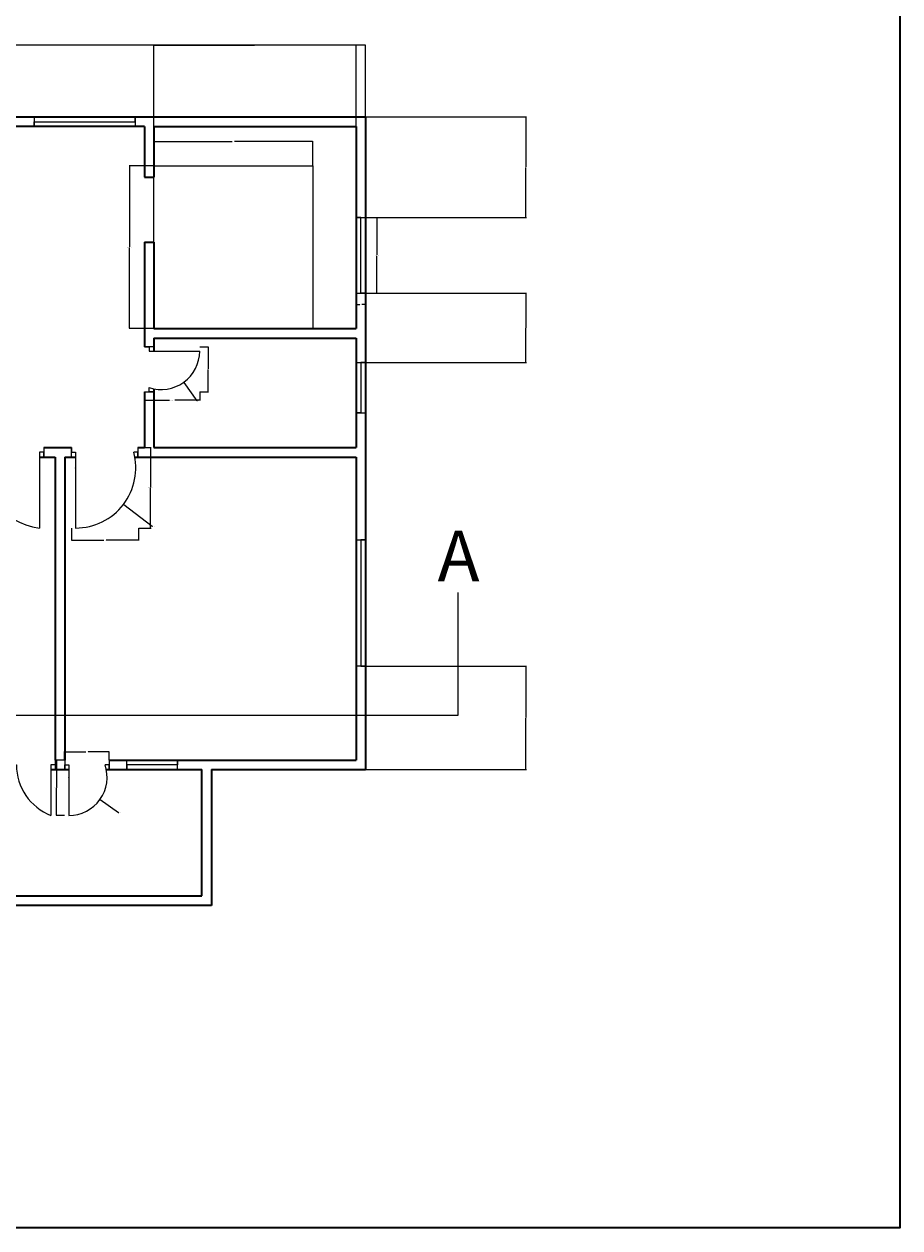
# Model space of a CAD drawing. Units: inches. Extents: x 2055 to 3558, y 1520 to 2888.
# Tile 6 of 8: x 3142 to 3558, y 1520 to 2092. Entities that reach past the tile are written whole.
import ezdxf

# ---------------------------------------------------------------- set-up
doc = ezdxf.new("R2010")
doc.units = ezdxf.units.IN
for name, color, linetype, lineweight in [('A-ANNO-DIMS', 2, 'Continuous', 18), ('A-ANNO-SYMB', 7, 'Continuous', 25), ('A-ANNO-TTLB', 7, 'Continuous', 35), ('A-DOOR', 3, 'Continuous', 18), ('A-FLOR-FIXT', 8, 'Continuous', 18), ('A-GLAZ', 4, 'Continuous', 18), ('A-WALL', 7, 'Continuous', 35)]:
    doc.layers.add(name, color=color, linetype=linetype, lineweight=lineweight)
doc.styles.get("Standard").update_dxf_attribs({"font": 'arial.ttf'})
doc.dimstyles.get("Standard").update_dxf_attribs({"dimtxt": 0.18, "dimasz": 0.18, "dimexe": 0.18, "dimexo": 0.0625, "dimgap": 0.09, "dimtad": 0, "dimtih": 1, "dimtoh": 1, "dimdec": 4, "dimzin": 0, "dimdsep": 46, "dimtxsty": 'Standard', "dimcen": 0.09, "dimadec": 0, "dimazin": 0, "dimtfac": 1, "dimtdec": 4, "dimtofl": 0, "dimtmove": 0, "dimatfit": 3, "dimfxl": 1, "dimtolj": 1, "dimtzin": 0, "dimarcsym": 0})

# ---------------------------------------------------------------- blocks, each defined once
blk = doc.blocks.new('DOOR-BATH-24-B')
for p, q in [((4.5, 21.32), (0, 21.32)), ((0, 21.32), (2.25, 21.32)), ((2.25, 21.32), (2.25, 19.32)), ((2.25, 19.32), (26.25, 19.32)), ((0, 0), (4.5, 0)), ((2.25, 0), (2.25, 2)), ((4.5, 0), (2.25, 0))]:
    blk.add_line(p, q)
blk.add_arc((8, 19.32), 18.25, 251.6403, 0)
blk = doc.blocks.new('DOOR-BED-36-F')
for p, q in [((0, 33.75), (0, 38.25)), ((0, 38.25), (0, 36)), ((0, 36), (2, 36)), ((2, 36), (2, 0)), ((31.57, 36), (29.57, 36)), ((31.57, 38.25), (31.57, 33.75)), ((31.57, 33.75), (31.57, 36))]:
    blk.add_line(p, q)
blk.add_arc((2, 28.56), 28.56, 270, 15.1117)
blk = doc.blocks.new('DOOR-BED-36-G')
for p, q in [((0, 38.25), (0, 33.75)), ((0, 33.75), (0, 36)), ((0, 36), (2, 36)), ((34.89, 36), (32.89, 36)), ((32.89, 36), (32.89, 0)), ((34.89, 38.25), (34.89, 33.75)), ((34.89, 33.75), (34.89, 36))]:
    blk.add_line(p, q)
blk.add_arc((38.42, 36), 36.42, 180, 261.253)
blk = doc.blocks.new('DOOR-VERANDA-24-A')
for p, q in [((0, 26.25), (0, 21.75)), ((0, 21.75), (0, 24)), ((0, 24), (2, 24)), ((2, 24), (2, 0)), ((21.18, 24), (19.18, 24)), ((21.18, 26.25), (21.18, 21.75)), ((21.18, 21.75), (21.18, 24))]:
    blk.add_line(p, q)
blk.add_arc((2, 18.15), 18.15, 270, 18.8194)
blk = doc.blocks.new('DOOR-VERANDA-24-B')
for p, q in [((0, 26.25), (0, 21.75)), ((0, 21.75), (0, 24)), ((0, 24), (2, 24)), ((20.42, 24), (18.42, 24)), ((18.42, 24), (18.42, 0)), ((20.42, 26.25), (20.42, 21.75))]:
    blk.add_line(p, q)
blk.add_arc((27.75, 24), 25.75, 180, 248.7547)
blk = doc.blocks.new('WIN-36')
for p, q in [((2.25, 36), (0, 36)), ((0, 36), (4.5, 36)), ((2.25, 0), (2.25, 36)), ((0, 0), (4.5, 0)), ((4.5, 0), (2.25, 0))]:
    blk.add_line(p, q)
blk = doc.blocks.new('WIN-24')
for p, q in [((0, 24), (4.5, 24)), ((4.5, 24), (2.25, 24)), ((2.25, 24), (2.25, 0)), ((2.25, 0), (0, 0)), ((0, 0), (4.5, 0))]:
    blk.add_line(p, q)
blk = doc.blocks.new('WIN-60-2')
for p, q in [((4.5, 60), (0, 60)), ((0, 60), (2.25, 60)), ((2.25, 60), (2.25, 0)), ((2.25, 0), (0, 0)), ((0, 0), (4.5, 0))]:
    blk.add_line(p, q)
blk = doc.blocks.new('WIN-48')
for p, q in [((0, 4.5), (0, 0)), ((0, 0), (0, 2.25)), ((0, 2.25), (48, 2.25)), ((48, 2.25), (48, 4.5)), ((48, 4.5), (48, 0))]:
    blk.add_line(p, q)
blk = doc.blocks.new('COUNTER-4')
for p, q in [((0, 77.26), (75.5, 77.26)), ((75.5, 77.26), (75.5, 0))]:
    blk.add_line(p, q)
blk = doc.blocks.new('VERANDA-PERIMETER')
for p, q in [((0, 0), (0, 64.5)), ((4.5, 64.5), (4.5, 4.5)), ((124.15, 4.5), (124.15, 64.5)), ((128.65, 64.5), (128.65, 4.5)), ((4.5, 0), (0, 0)), ((4.5, 4.5), (124.15, 4.5)), ((128.65, 0), (4.5, 0)), ((128.65, 4.5), (128.65, 0))]:
    blk.add_line(p, q)
blk = doc.blocks.new('*D42')
at = {"layer": 'A-ANNO-DIMS', "color": 0, "lineweight": -2, "transparency": 16777216}
for p, q in [((3304.06, 2000.28), (3309.58, 2000.28)), ((3309.4, 2000.1), (3309.4, 1982.46)), ((3309.4, 1964.46), (3309.4, 1982.1)), ((3304.06, 1964.28), (3309.58, 1964.28))]:
    blk.add_line(p, q, dxfattribs=at)
at = {"layer": 'A-ANNO-DIMS', "color": 0, "transparency": 16777216}
for points in [[(3309.37, 2000.1), (3309.43, 2000.1), (3309.4, 2000.28)], [(3309.37, 1964.46), (3309.43, 1964.46), (3309.4, 1964.28)]]:
    blk.add_solid(points, dxfattribs=at)
at = {"layer": 'Defpoints', "color": 0, "transparency": 16777216}
for p in [(3304, 2000.28), (3309.4, 2000.28), (3304, 1964.28)]:
    blk.add_point(p, dxfattribs=at)
at = {"layer": 'A-ANNO-DIMS', "color": 0, "transparency": 16777216, "insert": (3309.4, 1982.28), "char_height": 0.18, "attachment_point": 5}
blk.add_mtext('\\A1;WINDOW 36 TYP.', dxfattribs=at)
blk = doc.blocks.new('*D43')
at = {"layer": 'A-ANNO-DIMS', "color": 0, "lineweight": -2, "transparency": 16777216}
for p, q in [((3299.5, 1964.22), (3299.5, 1958.7)), ((3304, 1964.22), (3304, 1958.7)), ((3299.68, 1958.88), (3301.29, 1958.88)), ((3303.82, 1958.88), (3302.2, 1958.88))]:
    blk.add_line(p, q, dxfattribs=at)
at = {"layer": 'A-ANNO-DIMS', "color": 0, "transparency": 16777216}
for points in [[(3299.68, 1958.91), (3299.68, 1958.85), (3299.5, 1958.88)], [(3303.82, 1958.91), (3303.82, 1958.85), (3304, 1958.88)]]:
    blk.add_solid(points, dxfattribs=at)
at = {"layer": 'Defpoints', "color": 0, "transparency": 16777216}
for p in [(3299.5, 1964.28), (3304, 1964.28), (3304, 1958.88)]:
    blk.add_point(p, dxfattribs=at)
at = {"layer": 'A-ANNO-DIMS', "color": 0, "transparency": 16777216, "insert": (3301.75, 1958.88), "char_height": 0.18, "attachment_point": 5}
blk.add_mtext('\\A1;5 TYP.', dxfattribs=at)
blk = doc.blocks.new('*D68')
at = {"layer": 'A-ANNO-DIMS', "color": 0, "lineweight": -2, "transparency": 16777216}
for p, q in [((3199, 1917.43), (3199, 1913.38)), ((3225.25, 1917.43), (3225.25, 1913.38)), ((3199.18, 1913.56), (3210.81, 1913.56)), ((3225.07, 1913.56), (3213.43, 1913.56))]:
    blk.add_line(p, q, dxfattribs=at)
at = {"layer": 'A-ANNO-DIMS', "color": 0, "transparency": 16777216}
for points in [[(3199.18, 1913.59), (3199.18, 1913.53), (3199, 1913.56)], [(3225.07, 1913.59), (3225.07, 1913.53), (3225.25, 1913.56)]]:
    blk.add_solid(points, dxfattribs=at)
at = {"layer": 'Defpoints', "color": 0, "transparency": 16777216}
for p in [(3199, 1917.49), (3225.25, 1917.49), (3225.25, 1913.56)]:
    blk.add_point(p, dxfattribs=at)
at = {"layer": 'A-ANNO-DIMS', "color": 0, "transparency": 16777216, "insert": (3212.12, 1913.56), "char_height": 0.18, "attachment_point": 5}
blk.add_mtext('\\A1;BATH DOOR 26 TYP.', dxfattribs=at)
blk = doc.blocks.new('*D69')
at = {"layer": 'A-ANNO-DIMS', "color": 0, "lineweight": -2, "transparency": 16777216}
for p, q in [((3225.31, 1938.82), (3229.36, 1938.82)), ((3229.18, 1938.64), (3229.18, 1928.34)), ((3229.18, 1917.67), (3229.18, 1927.98)), ((3225.31, 1917.49), (3229.36, 1917.49))]:
    blk.add_line(p, q, dxfattribs=at)
at = {"layer": 'A-ANNO-DIMS', "color": 0, "transparency": 16777216}
for points in [[(3229.15, 1938.64), (3229.21, 1938.64), (3229.18, 1938.82)], [(3229.15, 1917.67), (3229.21, 1917.67), (3229.18, 1917.49)]]:
    blk.add_solid(points, dxfattribs=at)
at = {"layer": 'Defpoints', "color": 0, "transparency": 16777216}
for p in [(3225.25, 1938.82), (3229.18, 1938.82), (3225.25, 1917.49)]:
    blk.add_point(p, dxfattribs=at)
at = {"layer": 'A-ANNO-DIMS', "color": 0, "transparency": 16777216, "insert": (3229.18, 1928.16), "char_height": 0.18, "attachment_point": 5}
blk.add_mtext('\\A1;21 TYP.', dxfattribs=at)
blk = doc.blocks.new('*D78')
at = {"layer": 'A-ANNO-DIMS', "color": 0, "lineweight": -2, "transparency": 16777216}
for p, q in [((3196.25, 1891), (3202.11, 1891)), ((3201.93, 1890.82), (3201.93, 1872.06)), ((3201.93, 1852.93), (3201.93, 1871.69)), ((3196.25, 1852.75), (3202.11, 1852.75))]:
    blk.add_line(p, q, dxfattribs=at)
at = {"layer": 'A-ANNO-DIMS', "color": 0, "transparency": 16777216}
for points in [[(3201.9, 1890.82), (3201.96, 1890.82), (3201.93, 1891)], [(3201.9, 1852.93), (3201.96, 1852.93), (3201.93, 1852.75)]]:
    blk.add_solid(points, dxfattribs=at)
at = {"layer": 'Defpoints', "color": 0, "transparency": 16777216}
for p in [(3196.19, 1891), (3201.93, 1891), (3196.19, 1852.75)]:
    blk.add_point(p, dxfattribs=at)
at = {"layer": 'A-ANNO-DIMS', "color": 0, "transparency": 16777216, "insert": (3201.93, 1871.87), "char_height": 0.18, "attachment_point": 5}
blk.add_mtext('\\A1;BED DOOR 38 TYP.', dxfattribs=at)
blk = doc.blocks.new('*D79')
at = {"layer": 'A-ANNO-DIMS', "color": 0, "lineweight": -2, "transparency": 16777216}
for p, q in [((3164.3, 1852.69), (3164.3, 1846.83)), ((3196.19, 1852.69), (3196.19, 1846.83)), ((3164.48, 1847.01), (3179.72, 1847.01)), ((3196.01, 1847.01), (3180.77, 1847.01))]:
    blk.add_line(p, q, dxfattribs=at)
at = {"layer": 'A-ANNO-DIMS', "color": 0, "transparency": 16777216}
for points in [[(3164.48, 1847.04), (3164.48, 1846.98), (3164.3, 1847.01)], [(3196.01, 1847.04), (3196.01, 1846.98), (3196.19, 1847.01)]]:
    blk.add_solid(points, dxfattribs=at)
at = {"layer": 'Defpoints', "color": 0, "transparency": 16777216}
for p in [(3164.3, 1852.75), (3196.19, 1852.75), (3196.19, 1847.01)]:
    blk.add_point(p, dxfattribs=at)
at = {"layer": 'A-ANNO-DIMS', "color": 0, "transparency": 16777216, "insert": (3180.25, 1847.01), "char_height": 0.18, "attachment_point": 5}
blk.add_mtext('\\A1;32 TYP.', dxfattribs=at)
blk = doc.blocks.new('*D82')
at = {"layer": 'A-ANNO-DIMS', "color": 0, "lineweight": -2, "transparency": 16777216}
for p, q in [((3161.03, 1742.5), (3156.98, 1742.5)), ((3157.16, 1742.32), (3157.16, 1729.56)), ((3157.16, 1716.43), (3157.16, 1729.19)), ((3161.03, 1716.25), (3156.98, 1716.25))]:
    blk.add_line(p, q, dxfattribs=at)
at = {"layer": 'A-ANNO-DIMS', "color": 0, "transparency": 16777216}
for points in [[(3157.13, 1742.32), (3157.19, 1742.32), (3157.16, 1742.5)], [(3157.13, 1716.43), (3157.19, 1716.43), (3157.16, 1716.25)]]:
    blk.add_solid(points, dxfattribs=at)
at = {"layer": 'Defpoints', "color": 0, "transparency": 16777216}
for p in [(3157.16, 1742.5), (3161.09, 1742.5), (3161.09, 1716.25)]:
    blk.add_point(p, dxfattribs=at)
at = {"layer": 'A-ANNO-DIMS', "color": 0, "transparency": 16777216, "insert": (3157.16, 1729.37), "char_height": 0.18, "attachment_point": 5}
blk.add_mtext('\\A1;DOOR 26 TYP.', dxfattribs=at)
blk = doc.blocks.new('*D83')
at = {"layer": 'A-ANNO-DIMS', "color": 0, "lineweight": -2, "transparency": 16777216}
for p, q in [((3161.09, 1742.56), (3161.09, 1746.62)), ((3161.27, 1746.44), (3171.15, 1746.44)), ((3182.09, 1746.44), (3172.21, 1746.44)), ((3182.27, 1742.56), (3182.27, 1746.62))]:
    blk.add_line(p, q, dxfattribs=at)
at = {"layer": 'A-ANNO-DIMS', "color": 0, "transparency": 16777216}
for points in [[(3161.27, 1746.47), (3161.27, 1746.41), (3161.09, 1746.44)], [(3182.09, 1746.47), (3182.09, 1746.41), (3182.27, 1746.44)]]:
    blk.add_solid(points, dxfattribs=at)
at = {"layer": 'Defpoints', "color": 0, "transparency": 16777216}
for p in [(3182.27, 1746.44), (3161.09, 1742.5), (3182.27, 1742.5)]:
    blk.add_point(p, dxfattribs=at)
at = {"layer": 'A-ANNO-DIMS', "color": 0, "transparency": 16777216, "insert": (3171.68, 1746.44), "char_height": 0.18, "attachment_point": 5}
blk.add_mtext('\\A1;21 TYP.', dxfattribs=at)
blk = doc.blocks.new('*D112')
at = {"layer": 'A-ANNO-DIMS', "color": 0, "lineweight": -2, "transparency": 16777216}
for p, q in [((3203.43, 2024.76), (3191.73, 2024.76)), ((3191.91, 2024.58), (3191.91, 1986.31)), ((3191.91, 1947.68), (3191.91, 1985.95)), ((3203.43, 1947.5), (3191.73, 1947.5))]:
    blk.add_line(p, q, dxfattribs=at)
at = {"layer": 'A-ANNO-DIMS', "color": 0, "transparency": 16777216}
for points in [[(3191.88, 2024.58), (3191.94, 2024.58), (3191.91, 2024.76)], [(3191.88, 1947.68), (3191.94, 1947.68), (3191.91, 1947.5)]]:
    blk.add_solid(points, dxfattribs=at)
at = {"layer": 'Defpoints', "color": 0, "transparency": 16777216}
for p in [(3191.91, 2024.76), (3203.5, 2024.76), (3203.5, 1947.5)]:
    blk.add_point(p, dxfattribs=at)
at = {"layer": 'A-ANNO-DIMS', "color": 0, "transparency": 16777216, "insert": (3191.91, 1986.13), "char_height": 0.18, "attachment_point": 5}
blk.add_mtext('\\A1;COUNTER 77 TYP.', dxfattribs=at)
blk = doc.blocks.new('*D113')
at = {"layer": 'A-ANNO-DIMS', "color": 0, "lineweight": -2, "transparency": 16777216}
for p, q in [((3203.5, 2024.82), (3203.5, 2036.53)), ((3203.68, 2036.35), (3240.72, 2036.35)), ((3278.82, 2036.35), (3241.78, 2036.35)), ((3279, 2024.82), (3279, 2036.53))]:
    blk.add_line(p, q, dxfattribs=at)
at = {"layer": 'A-ANNO-DIMS', "color": 0, "transparency": 16777216}
for points in [[(3203.68, 2036.38), (3203.68, 2036.32), (3203.5, 2036.35)], [(3278.82, 2036.38), (3278.82, 2036.32), (3279, 2036.35)]]:
    blk.add_solid(points, dxfattribs=at)
at = {"layer": 'Defpoints', "color": 0, "transparency": 16777216}
for p in [(3279, 2036.35), (3203.5, 2024.76), (3279, 2024.76)]:
    blk.add_point(p, dxfattribs=at)
at = {"layer": 'A-ANNO-DIMS', "color": 0, "transparency": 16777216, "insert": (3241.25, 2036.35), "char_height": 0.18, "attachment_point": 5}
blk.add_mtext('\\A1;76 TYP.', dxfattribs=at)
blk = doc.blocks.new('*D133')
at = {"layer": 'A-ANNO-DIMS', "color": 0, "lineweight": -2, "transparency": 16777216}
for p, q in [((2791.5, 2048.06), (2791.5, 2082.28)), ((2791.68, 2082.1), (3047.35, 2082.1)), ((3303.82, 2082.1), (3048.14, 2082.1)), ((3304, 2048.06), (3304, 2082.28))]:
    blk.add_line(p, q, dxfattribs=at)
at = {"layer": 'A-ANNO-DIMS', "color": 0, "transparency": 16777216}
for points in [[(2791.68, 2082.13), (2791.68, 2082.07), (2791.5, 2082.1)], [(3303.82, 2082.13), (3303.82, 2082.07), (3304, 2082.1)]]:
    blk.add_solid(points, dxfattribs=at)
at = {"layer": 'Defpoints', "color": 0, "transparency": 16777216}
for p in [(3304, 2082.1), (2791.5, 2048), (3304, 2048)]:
    blk.add_point(p, dxfattribs=at)
at = {"layer": 'A-ANNO-DIMS', "color": 0, "transparency": 16777216, "insert": (3047.75, 2082.1), "char_height": 0.18, "attachment_point": 5}
blk.add_mtext('\\A1;512.5', dxfattribs=at)
blk = doc.blocks.new('*D139')
at = {"layer": 'A-ANNO-DIMS', "color": 0, "lineweight": -2, "transparency": 16777216}
for p, q in [((3203.5, 1947.56), (3203.5, 2082.28)), ((3203.68, 2082.1), (3251.28, 2082.1)), ((3299.32, 2082.1), (3251.71, 2082.1)), ((3299.5, 1947.56), (3299.5, 2082.28))]:
    blk.add_line(p, q, dxfattribs=at)
at = {"layer": 'A-ANNO-DIMS', "color": 0, "transparency": 16777216}
for points in [[(3203.68, 2082.13), (3203.68, 2082.07), (3203.5, 2082.1)], [(3299.32, 2082.13), (3299.32, 2082.07), (3299.5, 2082.1)]]:
    blk.add_solid(points, dxfattribs=at)
at = {"layer": 'Defpoints', "color": 0, "transparency": 16777216}
for p in [(3299.5, 2082.1), (3203.5, 1947.5), (3299.5, 1947.5)]:
    blk.add_point(p, dxfattribs=at)
at = {"layer": 'A-ANNO-DIMS', "color": 0, "transparency": 16777216, "insert": (3251.5, 2082.1), "char_height": 0.18, "attachment_point": 5}
blk.add_mtext('\\A1;96', dxfattribs=at)
blk = doc.blocks.new('*D140')
at = {"layer": 'A-ANNO-DIMS', "color": 0, "lineweight": -2, "transparency": 16777216}
for p, q in [((3304.06, 2048), (3380.4, 2048)), ((3380.22, 2047.82), (3380.22, 2024.32)), ((3380.22, 2000.46), (3380.22, 2023.96)), ((3304.06, 2000.28), (3380.4, 2000.28))]:
    blk.add_line(p, q, dxfattribs=at)
at = {"layer": 'A-ANNO-DIMS', "color": 0, "transparency": 16777216}
for points in [[(3380.19, 2047.82), (3380.25, 2047.82), (3380.22, 2048)], [(3380.19, 2000.46), (3380.25, 2000.46), (3380.22, 2000.28)]]:
    blk.add_solid(points, dxfattribs=at)
at = {"layer": 'Defpoints', "color": 0, "transparency": 16777216}
for p in [(3304, 2048), (3304, 2000.28), (3380.22, 2000.28)]:
    blk.add_point(p, dxfattribs=at)
at = {"layer": 'A-ANNO-DIMS', "color": 0, "transparency": 16777216, "insert": (3380.22, 2024.14), "char_height": 0.18, "attachment_point": 5}
blk.add_mtext('\\A1;47.72', dxfattribs=at)
blk = doc.blocks.new('*D141')
at = {"layer": 'A-ANNO-DIMS', "color": 0, "lineweight": -2, "transparency": 16777216}
for p, q in [((3304.06, 1964.28), (3380.4, 1964.28)), ((3380.22, 1964.1), (3380.22, 1948.03)), ((3380.22, 1931.6), (3380.22, 1947.67)), ((3304.06, 1931.42), (3380.4, 1931.42))]:
    blk.add_line(p, q, dxfattribs=at)
at = {"layer": 'A-ANNO-DIMS', "color": 0, "transparency": 16777216}
for points in [[(3380.19, 1964.1), (3380.25, 1964.1), (3380.22, 1964.28)], [(3380.19, 1931.6), (3380.25, 1931.6), (3380.22, 1931.42)]]:
    blk.add_solid(points, dxfattribs=at)
at = {"layer": 'Defpoints', "color": 0, "transparency": 16777216}
for p in [(3304, 1964.28), (3304, 1931.42), (3380.22, 1931.42)]:
    blk.add_point(p, dxfattribs=at)
at = {"layer": 'A-ANNO-DIMS', "color": 0, "transparency": 16777216, "insert": (3380.22, 1947.85), "char_height": 0.18, "attachment_point": 5}
blk.add_mtext('\\A1;32.86', dxfattribs=at)
blk = doc.blocks.new('*D142')
at = {"layer": 'A-ANNO-DIMS', "color": 0, "lineweight": -2, "transparency": 16777216}
for p, q in [((3304.06, 1787.23), (3380.4, 1787.23)), ((3380.22, 1787.05), (3380.22, 1762.8)), ((3380.22, 1738.18), (3380.22, 1762.43)), ((3304.06, 1738), (3380.4, 1738))]:
    blk.add_line(p, q, dxfattribs=at)
at = {"layer": 'A-ANNO-DIMS', "color": 0, "transparency": 16777216}
for points in [[(3380.19, 1787.05), (3380.25, 1787.05), (3380.22, 1787.23)], [(3380.19, 1738.18), (3380.25, 1738.18), (3380.22, 1738)]]:
    blk.add_solid(points, dxfattribs=at)
at = {"layer": 'Defpoints', "color": 0, "transparency": 16777216}
for p in [(3304, 1787.23), (3380.22, 1787.23), (3304, 1738)]:
    blk.add_point(p, dxfattribs=at)
at = {"layer": 'A-ANNO-DIMS', "color": 0, "transparency": 16777216, "insert": (3380.22, 1762.61), "char_height": 0.18, "attachment_point": 5}
blk.add_mtext('\\A1;49.23', dxfattribs=at)
blk = doc.blocks.new('*D177')
at = {"layer": 'A-ANNO-DIMS', "color": 0, "lineweight": -2, "transparency": 16777216}
for p, q in [((3166.21, 1881.31), (3166.39, 1881.31)), ((3166.3, 1881.22), (3166.3, 1881.4)), ((3202.58, 1853.53), (3189.12, 1863.83)), ((3202.76, 1853.53), (3202.58, 1853.53))]:
    blk.add_line(p, q, dxfattribs=at)
at = {"layer": 'A-ANNO-DIMS', "color": 0, "transparency": 16777216}
blk.add_solid([(3189.14, 1863.86), (3189.1, 1863.81), (3188.98, 1863.94)], dxfattribs=at)
at = {"layer": 'Defpoints', "color": 0, "transparency": 16777216}
for p in [(3166.3, 1881.31), (3188.98, 1863.94)]:
    blk.add_point(p, dxfattribs=at)
at = {"layer": 'A-ANNO-DIMS', "color": 0, "transparency": 16777216, "insert": (3203.31, 1853.53), "char_height": 0.18, "attachment_point": 5}
blk.add_mtext('\\A1;R28.556', dxfattribs=at)
blk = doc.blocks.new('*D183')
at = {"layer": 'A-ANNO-DIMS', "color": 0, "lineweight": -2, "transparency": 16777216}
for p, q in [((3206.9, 1936.82), (3207.08, 1936.82)), ((3206.99, 1936.73), (3206.99, 1936.91)), ((3224.08, 1913.14), (3217.78, 1921.87)), ((3224.26, 1913.14), (3224.08, 1913.14))]:
    blk.add_line(p, q, dxfattribs=at)
at = {"layer": 'A-ANNO-DIMS', "color": 0, "transparency": 16777216}
blk.add_solid([(3217.81, 1921.89), (3217.76, 1921.85), (3217.68, 1922.02)], dxfattribs=at)
at = {"layer": 'Defpoints', "color": 0, "transparency": 16777216}
for p in [(3206.99, 1936.82), (3217.68, 1922.02)]:
    blk.add_point(p, dxfattribs=at)
at = {"layer": 'A-ANNO-DIMS', "color": 0, "transparency": 16777216, "insert": (3224.75, 1913.14), "char_height": 0.18, "attachment_point": 5}
blk.add_mtext('\\A1;R18.25', dxfattribs=at)
blk = doc.blocks.new('*D184')
at = {"layer": 'A-ANNO-DIMS', "color": 0, "lineweight": -2, "transparency": 16777216}
for p, q in [((3163, 1734.4), (3163.18, 1734.4)), ((3163.09, 1734.31), (3163.09, 1734.49)), ((3186.71, 1717.5), (3178, 1723.73)), ((3186.89, 1717.5), (3186.71, 1717.5))]:
    blk.add_line(p, q, dxfattribs=at)
at = {"layer": 'A-ANNO-DIMS', "color": 0, "transparency": 16777216}
blk.add_solid([(3178.02, 1723.75), (3177.98, 1723.71), (3177.85, 1723.83)], dxfattribs=at)
at = {"layer": 'Defpoints', "color": 0, "transparency": 16777216}
for p in [(3163.09, 1734.4), (3177.85, 1723.83)]:
    blk.add_point(p, dxfattribs=at)
at = {"layer": 'A-ANNO-DIMS', "color": 0, "transparency": 16777216, "insert": (3187.43, 1717.5), "char_height": 0.18, "attachment_point": 5}
blk.add_mtext('\\A1;R18.146', dxfattribs=at)

msp = doc.modelspace()

# ---------------------------------------------------------------- linework, layer by layer
at = {"layer": 'A-ANNO-SYMB'}
for p, q in [((3348.0248, 1763.9223), (3348.0248, 1822.1362)), ((2735.2074, 1763.9223), (3348.0248, 1763.9223))]:
    msp.add_line(p, q, dxfattribs=at)
at = {"layer": 'A-ANNO-TTLB'}
msp.add_lwpolyline([(2054.7598, 2888.2545), (3557.8479, 2888.2545), (3557.8479, 1520.3256), (2054.7598, 1520.3256)], close=True, dxfattribs=at)
at = {"layer": 'A-WALL'}
for p, q in [((3136.1429, 2047.9995), (3303.9955, 2047.9995)), ((3303.9955, 2047.9995), (3303.9955, 1737.9995)), ((3198.9955, 2043.4995), (3134.679, 2043.4995)), ((3198.9955, 2043.4995), (3198.9955, 2019.4149)), ((3203.4955, 2043.4995), (3299.4955, 2043.4995)), ((3203.4955, 2043.4995), (3203.4955, 2019.4149)), ((3299.4955, 2043.4995), (3299.4955, 1947.4995)), ((3198.9955, 2019.4149), (3203.4955, 2019.4149)), ((3198.9955, 1988.6064), (3198.9955, 1938.8165)), ((3198.9955, 1988.6064), (3203.4955, 1988.6064)), ((3203.4955, 1988.6064), (3203.4955, 1947.4995)), ((3203.4955, 1947.4995), (3299.4955, 1947.4995)), ((3203.4955, 1942.9995), (3299.4955, 1942.9995)), ((3203.4955, 1942.9995), (3203.4955, 1936.8165)), ((3299.4955, 1942.9995), (3299.4955, 1890.9995)), ((3198.9955, 1917.4944), (3198.9955, 1890.9995)), ((3203.4955, 1918.9038), (3203.4955, 1890.9995)), ((3151.1389, 1890.9995), (3164.3033, 1890.9995)), ((3195.8714, 1890.9995), (3198.9955, 1890.9995)), ((3203.4955, 1890.9995), (3299.4955, 1890.9995)), ((3149.1389, 1886.4995), (3156.5947, 1886.4995)), ((3156.5947, 1886.4995), (3156.5947, 1742.4995)), ((3161.0947, 1886.4995), (3166.3033, 1886.4995)), ((3161.0947, 1886.4995), (3161.0947, 1742.4995)), ((3194.3824, 1886.4995), (3299.4955, 1886.4995)), ((3203.4955, 1886.4995), (3299.4955, 1886.4995)), ((3299.4955, 1886.4995), (3299.4955, 1742.4995)), ((3182.2709, 1742.4995), (3198.9955, 1742.4995)), ((3182.2709, 1742.4995), (3299.4955, 1742.4995)), ((3203.4955, 1742.4995), (3299.4955, 1742.4995)), ((3154.5947, 1737.9995), (3163.0947, 1737.9995)), ((3180.8795, 1737.9995), (3226.3119, 1737.9995)), ((3230.8119, 1737.9995), (3303.9955, 1737.9995))]:
    msp.add_line(p, q, dxfattribs=at)

# ---------------------------------------------------------------- block references
at = {"layer": 'A-DOOR'}
for name, p in [('DOOR-BATH-24-B', (3198.9958, 1917.494)), ('DOOR-BED-36-G', (3116.2538, 1852.749)), ('DOOR-BED-36-F', (3164.3038, 1852.749)), ('DOOR-VERANDA-24-B', (3136.1758, 1716.249)), ('DOOR-VERANDA-24-A', (3161.0948, 1716.249))]:
    msp.add_blockref(name, p, dxfattribs=at)
at = {"layer": 'A-FLOR-FIXT'}
msp.add_blockref('COUNTER-4', (3203.4958, 1947.499), dxfattribs=at)
at = {"layer": 'A-GLAZ'}
for name, p in [('WIN-48', (3146.6438, 2043.499)), ('WIN-36', (3299.4958, 1964.2795)), ('WIN-24', (3299.4958, 1907.4213))]:
    msp.add_blockref(name, p, dxfattribs=at)
at = {"layer": 'A-GLAZ', "extrusion": (0, 0, -1), "zscale": -1}
msp.add_blockref('WIN-60-2', (-3303.9951, 1787.2273), dxfattribs=at)
at = {"layer": 'A-GLAZ', "extrusion": (0, 0, -1), "zscale": -1, "rotation": 90}
msp.add_blockref('WIN-24', (-3190.6328, 1737.9998), dxfattribs=at)
at = {"layer": 'A-WALL'}
msp.add_blockref('VERANDA-PERIMETER', (3102.1657, 1673.499), dxfattribs=at)

# ---------------------------------------------------------------- texts
at = {"layer": 'A-ANNO-SYMB', "insert": (3338.2255, 1851.5041), "char_height": 24, "attachment_point": 1}
msp.add_mtext_dynamic_manual_height_columns('A', width=25.660893, gutter_width=12.5, heights=[0], dxfattribs=at)

# ---------------------------------------------------------------- dimensions: what is measured, and where the dimension line sits
at = {"layer": 'A-ANNO-DIMS'}
for base, p1, p2, override, picture, middle in [((3303.9955, 2082.0995), (2791.4955, 2047.9995), (3303.9955, 2047.9995), {"dimdec": 1, "dimlfac": 1, "dimrnd": 0, "dimzin": 0, "dimdsep": 46, "dimlunit": 2}, '*D133', (3047.7455, 2082.0995)), ((3299.4955, 2082.0995), (3203.4955, 1947.4995), (3299.4955, 1947.4995), {"dimdec": 0, "dimlfac": 1, "dimrnd": 0, "dimzin": 0, "dimdsep": 46, "dimlunit": 2}, '*D139', (3251.4955, 2082.0995))]:
    dim = msp.add_linear_dim(base=base, p1=p1, p2=p2, dimstyle='Standard', override=override, dxfattribs=at)
    dim.commit()
    dim.dimension.update_dxf_attribs({"geometry": picture, "text_midpoint": middle})
for base, p1, p2, picture, middle in [((3380.2248, 2000.2797), (3303.9955, 2047.9995), (3303.9955, 2000.2797), '*D140', (3380.2248, 2024.1396)), ((3380.2248, 1931.4216), (3303.9955, 1964.2797), (3303.9955, 1931.4216), '*D141', (3380.2248, 1947.8507)), ((3380.2248, 1787.2274), (3303.9955, 1737.9995), (3303.9955, 1787.2274), '*D142', (3380.2248, 1762.6135))]:
    dim = msp.add_linear_dim(base=base, p1=p1, p2=p2, angle=90, dimstyle='Standard', override={"dimdec": 2, "dimlfac": 1, "dimrnd": 0, "dimzin": 0, "dimdsep": 46, "dimlunit": 2}, dxfattribs=at)
    dim.commit()
    dim.dimension.update_dxf_attribs({"geometry": picture, "text_midpoint": middle})
for base, p1, p2, text, picture, middle in [((3279.0006, 2036.3483), (3203.4955, 2024.7593), (3279.0006, 2024.7593), '<> TYP.', '*D113', (3241.248, 2036.3483)), ((3303.9954753785, 1958.8796928064), (3299.4954753785, 1964.2796928064), (3303.9954753785, 1964.2796928064), '<> TYP.', '*D43', (3301.7454753785, 1958.8796928064)), ((3225.2455, 1913.5569), (3198.9955, 1917.4944), (3225.2455, 1917.4944), 'BATH DOOR <> TYP.', '*D68', (3212.1205, 1913.5569)), ((3196.1884, 1847.012), (3164.3033, 1852.7495), (3196.1884, 1852.7495), '<> TYP.', '*D79', (3180.2459, 1847.012)), ((3182.2709, 1746.437), (3161.0947, 1742.4995), (3182.2709, 1742.4995), '<> TYP.', '*D83', (3171.6828, 1746.437))]:
    dim = msp.add_linear_dim(base=base, p1=p1, p2=p2, text=text, dimstyle='Standard', override={"dimdec": 0, "dimlfac": 1, "dimrnd": 0, "dimzin": 0, "dimdsep": 46, "dimlunit": 2}, dxfattribs=at)
    dim.commit()
    dim.dimension.update_dxf_attribs({"geometry": picture, "text_midpoint": middle})
for base, p1, p2, text, picture, middle in [((3191.9065, 2024.7593), (3203.4955, 1947.4995), (3203.4955, 2024.7593), 'COUNTER <> TYP.', '*D112', (3191.9065, 1986.1294)), ((3309.3955, 2000.2797), (3303.9955, 1964.2797), (3303.9955, 2000.2797), 'WINDOW <> TYP.', '*D42', (3309.3955, 1982.2797)), ((3229.183, 1938.8165), (3225.2455, 1917.4944), (3225.2455, 1938.8165), '<> TYP.', '*D69', (3229.183, 1928.1555)), ((3201.9259, 1890.9995), (3196.1884, 1852.7495), (3196.1884, 1890.9995), 'BED DOOR <> TYP.', '*D78', (3201.9259, 1871.8745)), ((3157.1572, 1742.4995), (3161.0947, 1716.2495), (3161.0947, 1742.4995), 'DOOR <> TYP.', '*D82', (3157.1572, 1729.3745))]:
    dim = msp.add_linear_dim(base=base, p1=p1, p2=p2, angle=90, text=text, dimstyle='Standard', override={"dimdec": 0, "dimlfac": 1, "dimrnd": 0, "dimzin": 0, "dimdsep": 46, "dimlunit": 2}, dxfattribs=at)
    dim.commit()
    dim.dimension.update_dxf_attribs({"geometry": picture, "text_midpoint": middle})
for center, mpoint, override, picture, middle in [((3206.9943, 1936.8165), (3217.6757, 1922.0174), {"dimdec": 2, "dimlfac": 1, "dimrnd": 0, "dimzin": 0, "dimdsep": 46, "dimlunit": 2}, '*D183', (3224.7451, 1913.138)), ((3166.3033, 1881.305), (3188.9751, 1863.9439), {"dimdec": 3, "dimlfac": 1, "dimrnd": 0, "dimzin": 0, "dimdsep": 46, "dimlunit": 2}, '*D177', (3203.3079, 1853.5272)), ((3163.0947, 1734.3958), (3177.8512, 1723.8349), {"dimdec": 3, "dimlfac": 1, "dimrnd": 0, "dimzin": 0, "dimdsep": 46, "dimlunit": 2}, '*D184', (3187.4348, 1717.4983))]:
    dim = msp.add_radius_dim(center=center, mpoint=mpoint, dimstyle='Standard', override=override, dxfattribs=at)
    dim.commit()
    dim.dimension.update_dxf_attribs({"geometry": picture, "text_midpoint": middle, "dimtype": 164})

doc.saveas('drawing.dxf')
